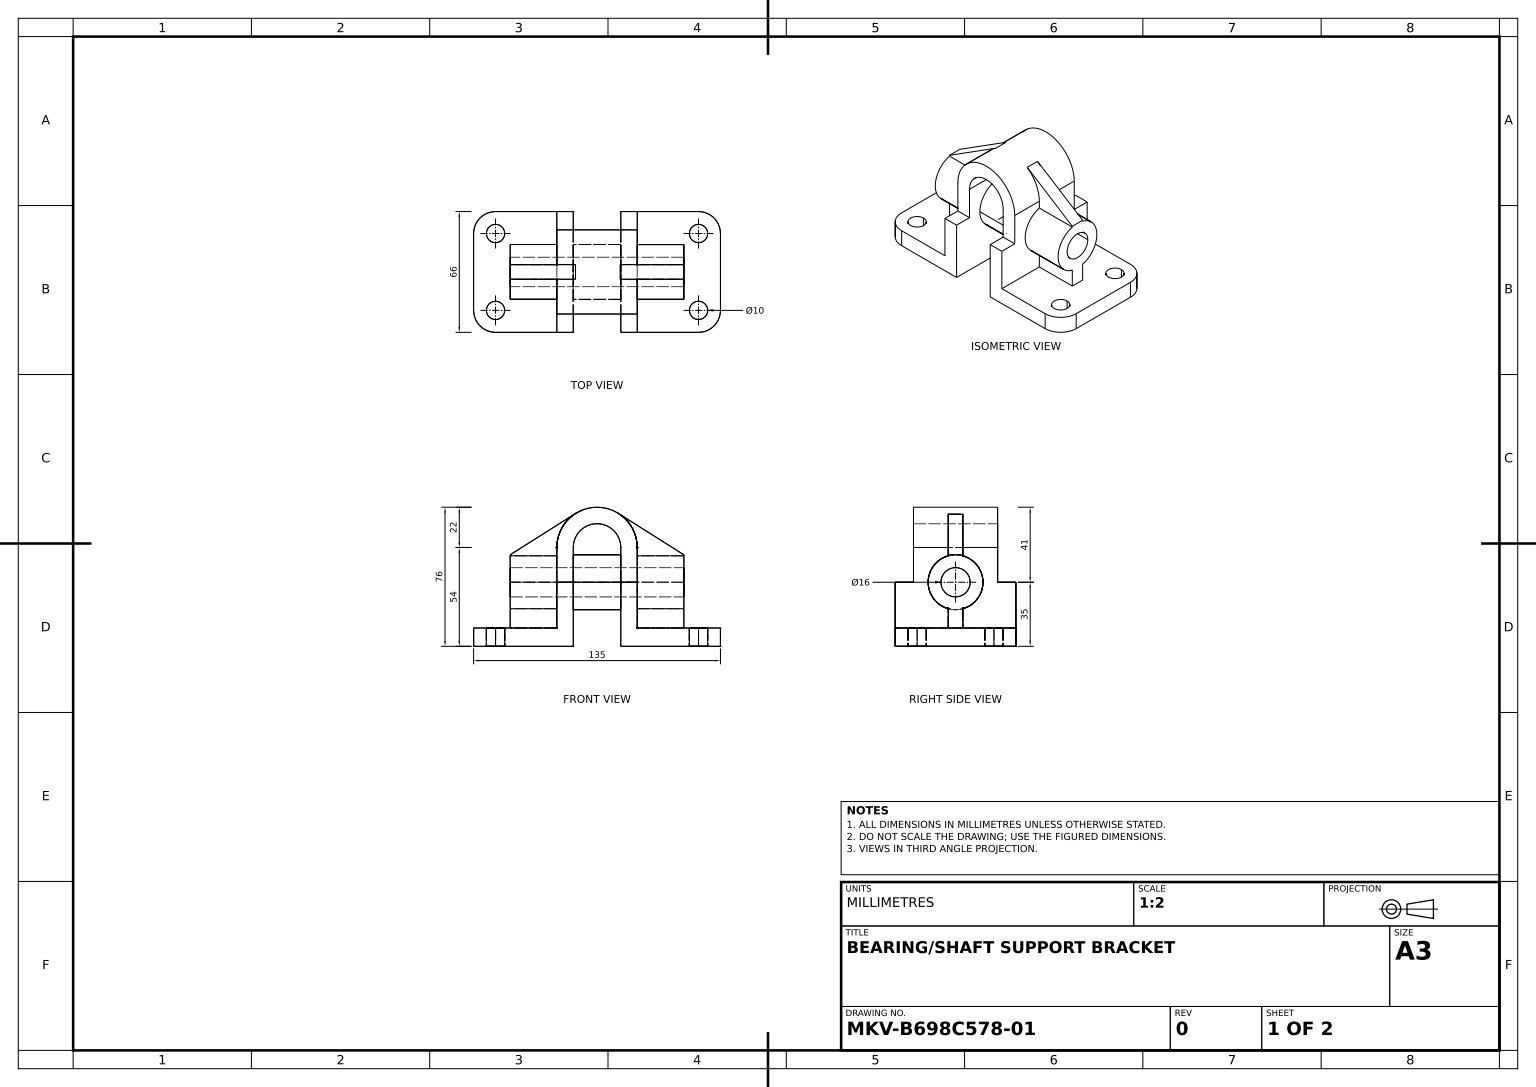
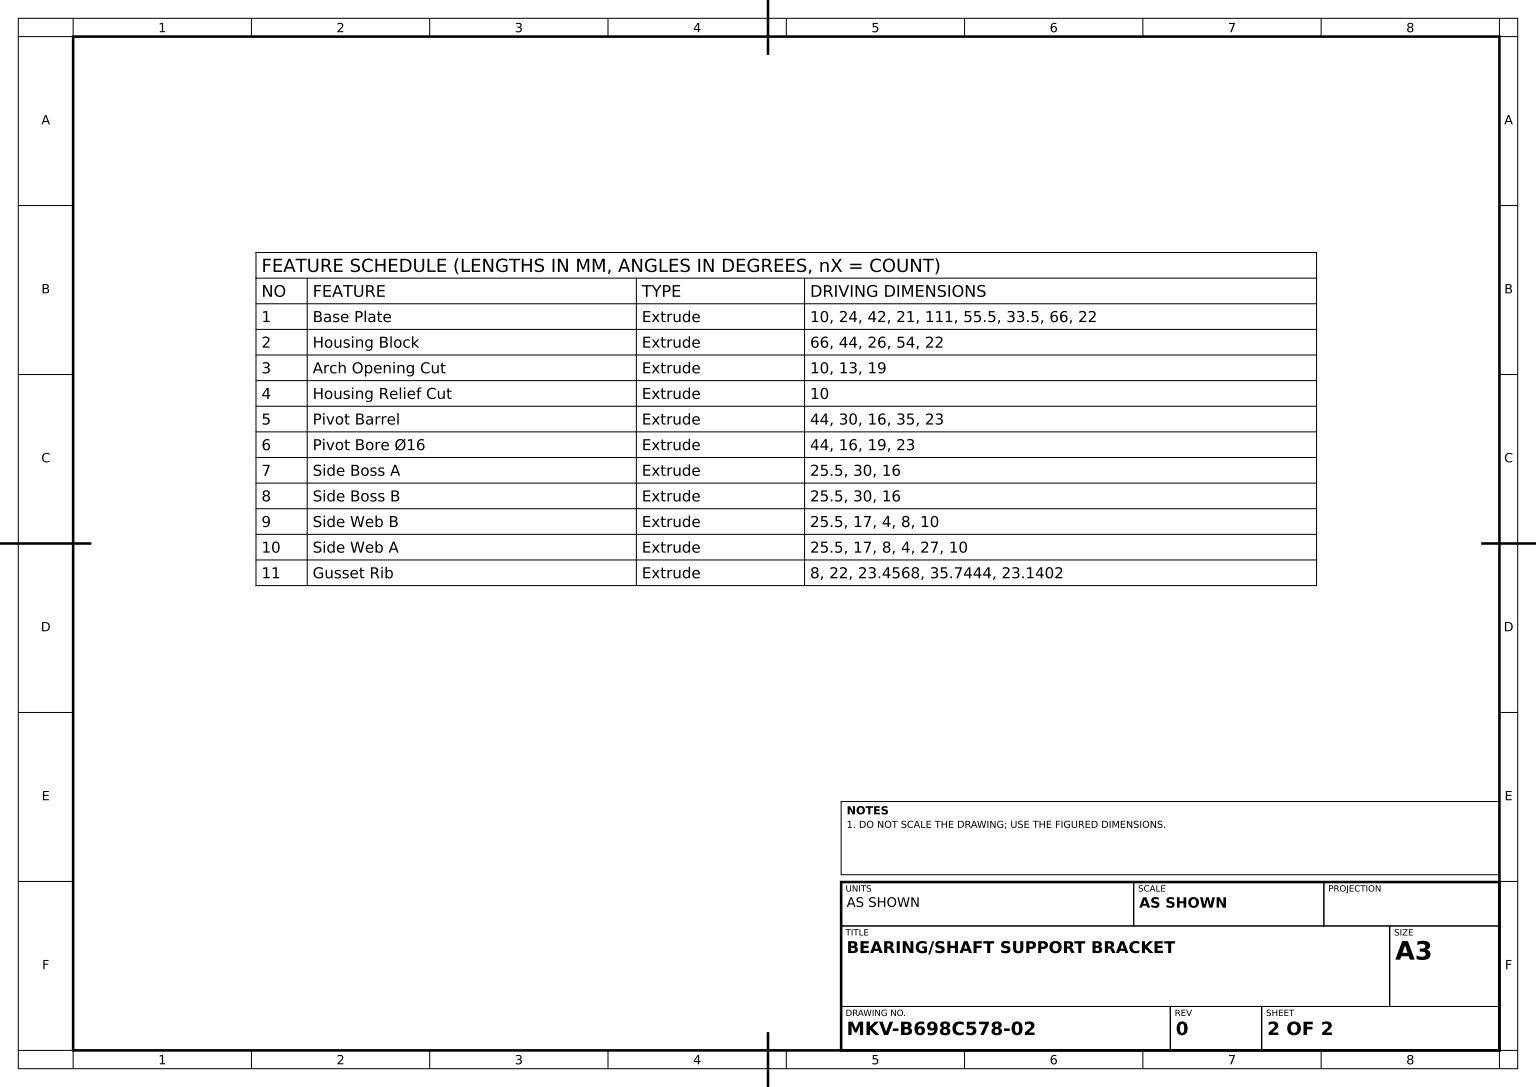
SolidWorks part; units mm, degrees
material "Plain Carbon Steel"
ref_plane "Front Plane" through (0, 0, 0) normal (0, 0, 1) x (1, 0, 0)
ref_plane "Top Plane" through (0, 0, 0) normal (0, 1, 0) x (1, 0, 0)
ref_plane "Right Plane" through (0, 0, 0) normal (1, 0, 0) x (0, 0, -1)
sketch "Base Plate Sketch" plane through (0, 0, 0) normal (0, 1, 0) x (1, 0, 0)
  line L0 (-55.5, 33) -> (-22, 33)
  line L1 (67.5, 21) -> (67.5, -21)
  line L2 (-22, 33) -> (-22, -33)
  line L3 (-22, -33) -> (-55.5, -33)
  line L4 (-67.5, 21) -> (-67.5, -21)
  line L5 (55.5, 33) -> (22, 33)
  line L6 (22, 33) -> (22, -33)
  line L7 (22, -33) -> (55.5, -33)
  arc A0 (-55.5, 33) -> (-67.5, 21) centre (-55.5, 21) ccw
  circle A1 centre (-55.5, 21) radius 5
  circle A2 centre (-55.5, -21) radius 5
  arc A3 (-67.5, -21) -> (-55.5, -33) centre (-55.5, -21) ccw
  arc A4 (67.5, 21) -> (55.5, 33) centre (55.5, 21) ccw
  circle A5 centre (55.5, 21) radius 5
  arc A6 (55.5, -33) -> (67.5, -21) centre (55.5, -21) ccw
  circle A7 centre (55.5, -21) radius 5
  dimension "D1" = 24
  dimension "D2" = 24
  dimension "D3" = 10
  dimension "D4" = 10
  dimension "D5" = 24
  dimension "D6" = 10
  dimension "D7" = 10
  dimension "D8" = 24
  dimension "D9" = 42
  dimension "D10" = 42
  dimension "D11" = 21
  dimension "D12" = 21
  dimension "D13" = 111
  dimension "D14" = 111
  dimension "D15" = 55.5
  dimension "D16" = 55.5
  dimension "D17" = 33.5
  dimension "D18" = 42
  dimension "D19" = 66
  dimension "D20" = 42
  dimension "D21" = 22
extrude "Base Plate" add sketch "Base Plate Sketch" along normal blind 10
sketch "Housing Block Sketch" plane through (0, 0, 33) normal (0, 0, 1) x (1, 0, 0)
  line L0 (22, 0) -> (55.5, 0) construction
  line L1 (-22, 54) -> (-22, 10)
  line L2 (-22, 10) -> (-22, 0)
  line L3 (-22, 0) -> (-13, 0)
  line L4 (-13, 0) -> (-13, 54)
  line L5 (13, 54) -> (13, 0)
  line L6 (13, 0) -> (22, 0)
  line L7 (22, 0) -> (22, 54)
  arc A0 (22, 54) -> (-22, 54) centre (0, 54) ccw
  arc A1 (13, 54) -> (-13, 54) centre (0, 54) ccw
  dimension "D1" = 44
  dimension "D2" = 26
  dimension "D3" = 54
  dimension "D4" = 22
extrude "Housing Block" add sketch "Housing Block Sketch" against normal blind 66
sketch "Arch Opening Sketch" plane through (0, 0, 33) normal (0, 0, 1) x (1, 0, 0)
  line L1 (13, 54) -> (13, 0) construction
  line L2 (13, 35) -> (22, 35)
  line L3 (22, 10) -> (22, 54) construction
  line L5 (13, 0) -> (55.5, 0) construction
  line L6 (22, 0) -> (13, 0)
  line L7 (-13, 35) -> (-22, 35)
  line L8 (-13, 0) -> (-13, 54) construction
  line L9 (-22, 54) -> (-22, 10) construction
  line L10 (-22, 35) -> (-22, 54)
  line L11 (-13, 35) -> (-13, 54)
  line L12 (13, 54) -> (13, 35)
  line L13 (22, 54) -> (22, 35)
  arc A0 (-22, 54) -> (22, 54) centre (0, 54) cw
  arc A1 (-13, 54) -> (13, 54) centre (0, 54) cw
  arc A2 (13, 54) -> (-13, 54) centre (0, 54) ccw construction
  line M6 (22, 10) -> (22, 54)
  arc M7 (22, 54) -> (-22, 54) centre (0, 54) ccw
  line M8 (-22, 54) -> (-22, 10)
  line M12 (-13, 0) -> (-13, 54)
  arc M13 (-13, 54) -> (13, 54) centre (0, 54) cw
  line M14 (13, 54) -> (13, 0)
  dimension "D1" = 13
  dimension "D2" = 19
extrude "Arch Opening Cut" cut sketch "Arch Opening Sketch" against normal blind 10 contours L7 L2 M12 M13 M14 M6 M7 M8
sketch "Housing Relief Sketch" plane through (0, 0, -33) normal (0, 0, -1) x (-1, 0, 0)
  line L1 (-13, 54) -> (-13, 0) construction
  line L2 (-13, 35) -> (-22, 35)
  line L3 (-22, 35) -> (-22, 54)
  line L4 (-13, 54) -> (-13, 35)
  line L5 (13, 54) -> (13, 35)
  line L6 (13, 35) -> (22, 35)
  line L7 (22, 54) -> (22, 10) construction
  line L8 (22, 35) -> (22, 54)
  arc A0 (-22, 54) -> (22, 54) centre (0, 54) cw
  arc A1 (-13, 54) -> (13, 54) centre (0, 54) cw
  arc A2 (13, 54) -> (-13, 54) centre (0, 54) ccw construction
extrude "Housing Relief Cut" cut sketch "Housing Relief Sketch" against normal blind 10
sketch "Pivot Barrel Sketch" plane through (-22, 0, 0) normal (-1, 0, 0) x (0, 0, 1)
  line L0 (-21, 0) -> (21, 0) construction
  line L1 (23, 54) -> (23, 35) construction
  circle A0 centre (0, 35) radius 15
  circle A1 centre (0, 35) radius 8
  dimension "D1" = 30
  dimension "D2" = 16
  dimension "D3" = 35
  dimension "D4" = 23
extrude "Pivot Barrel" add sketch "Pivot Barrel Sketch" against normal blind 44
sketch "Pivot Bore Sketch" plane through (-22, 0, 0) normal (-1, 0, 0) x (0, 0, 1)
  line L0 (-23, 54) -> (23, 54) construction
  line L1 (23, 54) -> (23, 35) construction
  circle A1 centre (0, 35) radius 8
  dimension "D1" = 16
  dimension "D2" = 19
  dimension "D3" = 23
extrude "Pivot Bore Ø16" cut sketch "Pivot Bore Sketch" against normal blind 44
sketch "Side Boss A Sketch" plane through (-22, 0, 0) normal (-1, 0, 0) x (0, 0, 1)
  circle A0 centre (0, 35) radius 8
  circle A1 centre (0, 35) radius 15
  dimension "D1" = 30
  dimension "D2" = 16
extrude "Side Boss A" add sketch "Side Boss A Sketch" along normal blind 25.5
sketch "Side Boss B Sketch" plane through (22, 0, 0) normal (1, 0, 0) x (0, 0, -1)
  circle A0 centre (0, 35) radius 8
  circle A1 centre (0, 35) radius 15
  dimension "D1" = 30
  dimension "D2" = 16
extrude "Side Boss B" add sketch "Side Boss B Sketch" along normal blind 25.5
sketch "Side Web B Sketch" plane through (47.5, 0, 0) normal (1, 0, 0) x (0, 0, -1)
  line L2 (-4, 27) -> (-4, 10)
  line L3 (4, 27) -> (4, 10)
  line L4 (-4, 27) -> (4, 27)
  line L5 (4, 27) -> (4, 10)
  line L6 (4, 10) -> (-4, 10)
  circle M6 centre (0, 35) radius 15
  dimension "D1" = 17
  dimension "D3" = 17
  dimension "D2" = 4
  dimension "D4" = 8
  dimension "D5" = 10
extrude "Side Web B" add sketch "Side Web B Sketch" against normal blind 25.5 contours L6 L3 L2 M6 | L4 L2 L3 M6
sketch "Side Web A Sketch" plane through (-47.5, 0, 0) normal (-1, 0, 0) x (0, 0, 1)
  line L2 (-4, 27) -> (-4, 10)
  line L3 (4, 27) -> (4, 10)
  line L4 (-4, 27) -> (4, 27)
  line L5 (-4, 10) -> (4, 10)
  dimension "D1" = 17
  dimension "D3" = 17
  dimension "D2" = 8
  dimension "D4" = 4
  dimension "D5" = 27
  dimension "D6" = 10
extrude "Side Web A" add sketch "Side Web A Sketch" against normal blind 25.5
ref_plane "Plane1" through (0, 0, 0) normal (0, 0, 1) x (1, 0, 0)
sketch "Gusset Rib Sketch" plane through (0, 0, 0) normal (0, 0, 1) x (1, 0, 0)
  line L0 (-47.5, 50) -> (-47.5, 44)
  line L1 (-47.5, 50) -> (-47.5, 20.5432) construction
  line L2 (-47.5, 44) -> (-22, 44)
  line L3 (47.5, 20.5432) -> (47.5, 50) construction
  line L4 (-47.5, 50) -> (-11.7556, 72.5958)
  line L5 (-22, 44) -> (-22, 54)
  line L6 (22, 54) -> (22, 44)
  line L7 (22, 20.5432) -> (22, 50) construction
  line L8 (47.5, 44) -> (47.5, 50)
  line L9 (22, 44) -> (47.5, 44)
  line L10 (-47.5, 20.5432) -> (-22, 20.5432) construction
  line L11 (47.5, 50) -> (10.8468, 73.1402)
  arc A0 (22, 54) -> (-22, 54) centre (0, 54) ccw construction
  arc A1 (-22, 54) -> (22, 54) centre (0, 54) cw
  dimension "D1" = 22
  dimension "D2" = 23.4568
  dimension "D3" = 23.1402
  dimension "D4" = 35.7444
extrude "Gusset Rib" add sketch "Gusset Rib Sketch" along normal mid plane 8 contours L5 A1 L4 L0 L2 | L11 A1 L6 L9 L8
